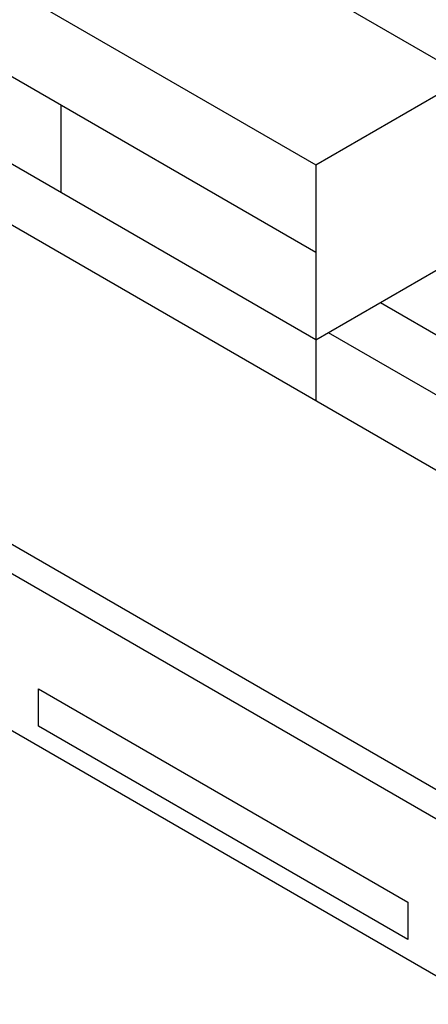
# Model space of a CAD drawing. Units: inches. Extents: x 5770 to 11891, y 3254 to 6808.
# Tile 8 of 15: x 6034 to 6048, y 3403 to 3436. Entities that reach past the tile are written whole.
import ezdxf

# ---------------------------------------------------------------- set-up
doc = ezdxf.new("R2010")
doc.units = ezdxf.units.IN
doc.layers.add('A-FURN', color=8, linetype='Continuous', lineweight=25)
doc.layers.add('A-GLAZ', color=4, linetype='Continuous', lineweight=25)

msp = doc.modelspace()

# ---------------------------------------------------------------- linework, layer by layer
at = {"layer": 'A-FURN'}
for p, q in [((5975.971, 3462.811), (6056.394, 3416.379)), ((5975.971, 3451.863), (6059.32, 3403.741)), ((5975.971, 3450.863), (6059.32, 3402.741)), ((6016.362, 3447.572), (6044.169, 3431.517)), ((5979.292, 3443.56), (6059.32, 3397.356)), ((6044.169, 3428.517), (6023.639, 3440.37)), ((6044.169, 3425.517), (6024.15, 3437.075)), ((6044.169, 3431.517), (6049.365, 3434.517)), ((6035.428, 3433.564), (6035.428, 3430.564)), ((6044.169, 3431.517), (6044.169, 3423.437)), ((6044.169, 3425.517), (6049.365, 3428.517)), ((6046.383, 3426.796), (6051.234, 3423.996)), ((6044.597, 3425.765), (6052.561, 3421.167)), ((6034.659, 3413.56), (6047.324, 3406.248)), ((6034.659, 3412.272), (6034.659, 3413.56)), ((6047.324, 3404.96), (6034.659, 3412.272)), ((6047.324, 3406.248), (6047.324, 3404.96))]:
    msp.add_line(p, q, dxfattribs=at)
at = {"layer": 'A-GLAZ'}
msp.add_line((6007.795, 3458.517), (6049.365, 3434.517), dxfattribs=at)

doc.saveas('drawing.dxf')
